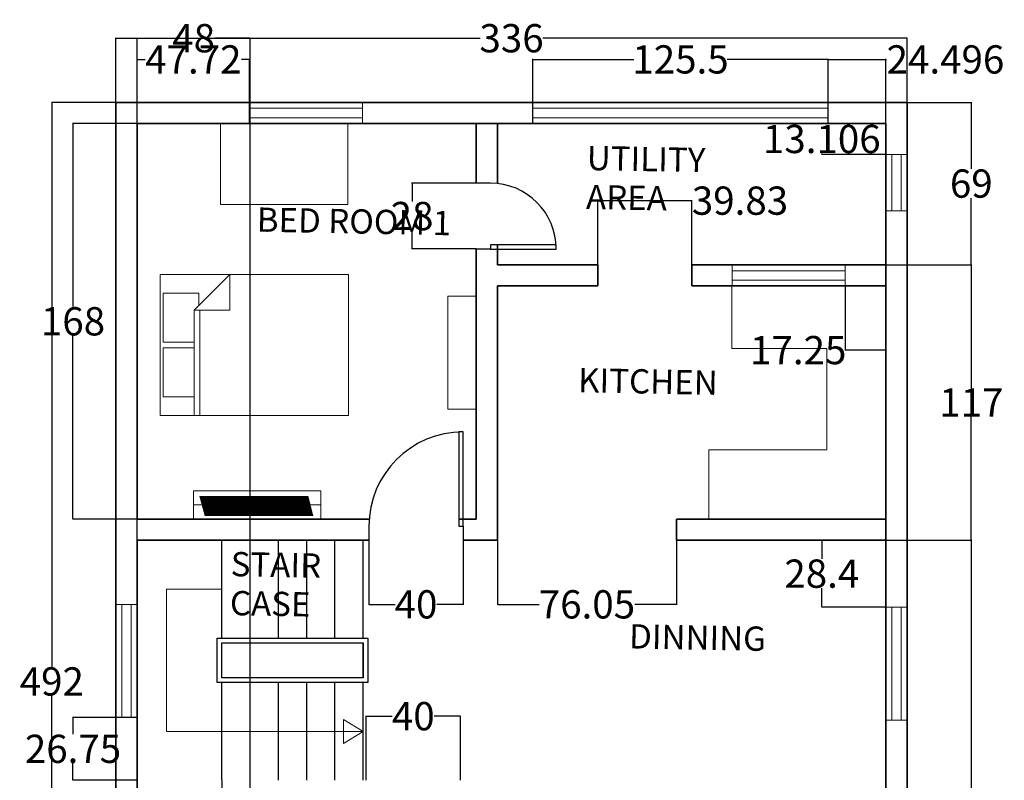
# Model space of a CAD drawing. Units: inches. Extents: x 424 to 1593, y 6 to 578.
# Tile 2 of 4: x 519 to 937, y 255 to 578. Entities that reach past the tile are written whole.
import ezdxf

# ---------------------------------------------------------------- set-up
doc = ezdxf.new("R2010")
doc.units = ezdxf.units.IN
doc.header["$MEASUREMENT"] = 0
for name, color, linetype, lineweight in [('A-ANNO-DIMS', 2, 'Continuous', 18), ('A-ANNO-SYMB', 2, 'Continuous', 18), ('A-AREA-IDEN', 7, 'Continuous', 18), ('A-DOOR', 3, 'Continuous', 25), ('A-FLOR-CASE', 9, 'Continuous', 18), ('A-FLOR-CASE-PATT', 252, 'Continuous', 13), ('A-FLOR-STRS', 7, 'Continuous', 25), ('A-FURN', 8, 'Continuous', 18), ('A-GLAZ', 4, 'Continuous', 18), ('A-WALL', 7, 'Continuous', 35)]:
    doc.layers.add(name, color=color, linetype=linetype, lineweight=lineweight)
doc.styles.get("Standard").update_dxf_attribs({"font": 'arial.ttf'})
doc.dimstyles.get("Standard").update_dxf_attribs({"dimtxt": 12, "dimasz": 0.18, "dimexe": 0.18, "dimexo": 0.0625, "dimgap": 0.09, "dimtad": 0, "dimtih": 1, "dimtoh": 1, "dimdec": 0, "dimzin": 0, "dimdsep": 46, "dimlunit": 3, "dimtxsty": 'Standard', "dimcen": 0.09, "dimadec": 0, "dimazin": 0, "dimtfac": 1, "dimtdec": 0, "dimtofl": 0, "dimtmove": 0, "dimatfit": 3, "dimfxl": 1, "dimtolj": 1, "dimtzin": 0, "dimarcsym": 0})

# ---------------------------------------------------------------- blocks, each defined once
blk = doc.blocks.new('Bed - Queen')
for p, q in [((0, -80.00003), (0, 0)), ((0, 0), (59.99999, 0)), ((59.99999, 0), (59.99999, -80.00003)), ((7.99999, -1.2), (28.79998, -1.2)), ((7.99999, -14.4), (7.99999, -1.2)), ((28.79998, -1.2), (28.79998, -14.4)), ((31.19999, -1.2), (51.99999, -1.2)), ((31.19999, -14.4), (31.19999, -1.2)), ((51.99999, -1.2), (51.99999, -16.4)), ((0, -14.4), (44.8, -14.4)), ((59.99999, -29.6), (44.8, -14.4)), ((44.8, -14.4), (44.8, -29.6)), ((51.99999, -16.4), (46.79936, -16.4)), ((44.8, -16.8), (0, -16.8)), ((44.8, -29.6), (59.99999, -29.6)), ((59.99999, -80.00003), (0, -80.00003))]:
    blk.add_line(p, q)
blk = doc.blocks.new('*U3')
for p, q in [((0, 0), (0, -6)), ((-40, 0), (-40, -6))]:
    blk.add_line(p, q)
blk.add_lwpolyline([(0, 0), (0, 40), (-1.75, 40), (-1.75, 0)], close=True)
blk.add_arc((0, 0), 40, 90, 180)
blk = doc.blocks.new('*U5')
for p, q in [((0, 0), (0, 6)), ((28, 0), (28, 6))]:
    blk.add_line(p, q)
blk.add_lwpolyline([(0, 0), (0, -28), (1.75, -28), (1.75, 0)], close=True)
blk.add_arc((0, 0), 28, 270, 0)
blk = doc.blocks.new('WIN-48IN')
for p, q in [((2.5, 48), (2.5, 0)), ((6.5, 48), (6.5, 0))]:
    blk.add_line(p, q)
blk.add_lwpolyline([(0, 48), (9, 48), (9, 0), (0, 0)], close=True)
blk = doc.blocks.new('WIN-24IN')
for p, q in [((2.5, 0), (2.5, 24)), ((6.5, 0), (6.5, 24))]:
    blk.add_line(p, q)
blk.add_lwpolyline([(9, 0), (0, 0), (0, 24), (9, 24)], close=True)
blk = doc.blocks.new('STAIR-RETURN-102IN')
for p, q in [((2, 60.44), (2, 102)), ((14, 60.44), (14, 102)), ((26, 60.44), (26, 102)), ((38, 60.44), (38, 102)), ((50, 60.44), (50, 102)), ((62, 60.44), (62, 102)), ((2, 43.56), (2, 58.44)), ((62, 43.56), (62, 58.44)), ((2, 0), (2, 41.56)), ((14, 0), (14, 41.56)), ((26, 0), (26, 41.56)), ((38, 0), (38, 41.56)), ((50, 0), (50, 41.56)), ((62, 0), (62, 41.56))]:
    blk.add_line(p, q)
for points in [[(0, 60.44), (64, 60.44), (64, 41.56), (0, 41.56)], [(2, 58.44), (62, 58.44), (62, 43.56), (2, 43.56)]]:
    blk.add_lwpolyline(points, close=True)
blk = doc.blocks.new('CASEWORK-48X12')
blk.add_lwpolyline([(12, 48), (0, 48), (0, 0), (12, 0)], close=True)
blk = doc.blocks.new('*D22')
at = {"layer": 'A-ANNO-DIMS', "color": 0, "lineweight": -2, "transparency": 16777216}
for p, q in [((559.72, 542.59), (559.72, 569.96)), ((559.9, 569.78), (714.38, 569.78)), ((895.54, 569.78), (741.05, 569.78)), ((895.72, 542.59), (895.72, 569.96))]:
    blk.add_line(p, q, dxfattribs=at)
at = {"layer": 'A-ANNO-DIMS', "color": 0, "transparency": 16777216}
for points in [[(559.9, 569.81), (559.9, 569.75), (559.72, 569.78)], [(895.54, 569.81), (895.54, 569.75), (895.72, 569.78)]]:
    blk.add_solid(points, dxfattribs=at)
at = {"layer": 'Defpoints', "color": 0, "transparency": 16777216}
for p in [(895.72, 569.78), (559.72, 542.53), (895.72, 542.53)]:
    blk.add_point(p, dxfattribs=at)
at = {"layer": 'A-ANNO-DIMS', "color": 0, "transparency": 16777216, "insert": (727.72, 569.78), "char_height": 12, "attachment_point": 5}
blk.add_mtext('\\A1;336', dxfattribs=at)
blk = doc.blocks.new('*D23')
at = {"layer": 'A-ANNO-DIMS', "color": 0, "lineweight": -2, "transparency": 16777216}
for p, q in [((559.65, 542.53), (532.29, 542.53)), ((532.47, 542.35), (532.47, 302.75)), ((532.47, 50.71), (532.47, 290.31)), ((559.65, 50.53), (532.29, 50.53))]:
    blk.add_line(p, q, dxfattribs=at)
at = {"layer": 'A-ANNO-DIMS', "color": 0, "transparency": 16777216}
for points in [[(532.44, 542.35), (532.5, 542.35), (532.47, 542.53)], [(532.44, 50.71), (532.5, 50.71), (532.47, 50.53)]]:
    blk.add_solid(points, dxfattribs=at)
at = {"layer": 'Defpoints', "color": 0, "transparency": 16777216}
for p in [(532.47, 542.53), (559.72, 542.53), (559.72, 50.53)]:
    blk.add_point(p, dxfattribs=at)
at = {"layer": 'A-ANNO-DIMS', "color": 0, "transparency": 16777216, "insert": (532.47, 296.53), "char_height": 12, "attachment_point": 5}
blk.add_mtext('\\A1;492', dxfattribs=at)
blk = doc.blocks.new('*D27')
at = {"layer": 'A-ANNO-DIMS', "color": 0, "lineweight": -2, "transparency": 16777216}
for p, q in [((568.65, 533.53), (541.29, 533.53)), ((541.47, 533.35), (541.47, 455.75)), ((541.47, 365.71), (541.47, 443.31)), ((568.65, 365.53), (541.29, 365.53))]:
    blk.add_line(p, q, dxfattribs=at)
at = {"layer": 'A-ANNO-DIMS', "color": 0, "transparency": 16777216}
for points in [[(541.44, 533.35), (541.5, 533.35), (541.47, 533.53)], [(541.44, 365.71), (541.5, 365.71), (541.47, 365.53)]]:
    blk.add_solid(points, dxfattribs=at)
at = {"layer": 'Defpoints', "color": 0, "transparency": 16777216}
for p in [(541.47, 533.53), (568.72, 533.53), (568.72, 365.53)]:
    blk.add_point(p, dxfattribs=at)
at = {"layer": 'A-ANNO-DIMS', "color": 0, "transparency": 16777216, "insert": (541.47, 449.53), "char_height": 12, "attachment_point": 5}
blk.add_mtext('\\A1;168', dxfattribs=at)
blk = doc.blocks.new('*D29')
at = {"layer": 'A-ANNO-DIMS', "color": 0, "lineweight": -2, "transparency": 16777216}
for p, q in [((886.78, 356.53), (923.15, 356.53)), ((922.97, 356.35), (922.97, 239.75)), ((922.97, 110.71), (922.97, 227.31)), ((895.78, 110.53), (923.15, 110.53))]:
    blk.add_line(p, q, dxfattribs=at)
at = {"layer": 'A-ANNO-DIMS', "color": 0, "transparency": 16777216}
for points in [[(922.94, 356.35), (923, 356.35), (922.97, 356.53)], [(922.94, 110.71), (923, 110.71), (922.97, 110.53)]]:
    blk.add_solid(points, dxfattribs=at)
at = {"layer": 'Defpoints', "color": 0, "transparency": 16777216}
for p in [(886.72, 356.53), (922.97, 356.53), (895.72, 110.53)]:
    blk.add_point(p, dxfattribs=at)
at = {"layer": 'A-ANNO-DIMS', "color": 0, "transparency": 16777216, "insert": (922.97, 233.53), "char_height": 12, "attachment_point": 5}
blk.add_mtext('\\A1;246', dxfattribs=at)
blk = doc.blocks.new('*D30')
at = {"layer": 'A-ANNO-DIMS', "color": 0, "lineweight": -2, "transparency": 16777216}
for p, q in [((886.78, 473.53), (923.15, 473.53)), ((922.97, 473.35), (922.97, 421.14)), ((922.97, 356.71), (922.97, 408.92)), ((886.78, 356.53), (923.15, 356.53))]:
    blk.add_line(p, q, dxfattribs=at)
at = {"layer": 'A-ANNO-DIMS', "color": 0, "transparency": 16777216}
for points in [[(922.94, 473.35), (923, 473.35), (922.97, 473.53)], [(922.94, 356.71), (923, 356.71), (922.97, 356.53)]]:
    blk.add_solid(points, dxfattribs=at)
at = {"layer": 'Defpoints', "color": 0, "transparency": 16777216}
for p in [(886.72, 473.53), (922.97, 473.53), (886.72, 356.53)]:
    blk.add_point(p, dxfattribs=at)
at = {"layer": 'A-ANNO-DIMS', "color": 0, "transparency": 16777216, "insert": (922.97, 415.03), "char_height": 12, "attachment_point": 5}
blk.add_mtext('\\A1;117', dxfattribs=at)
blk = doc.blocks.new('*D31')
at = {"layer": 'A-ANNO-DIMS', "color": 0, "lineweight": -2, "transparency": 16777216}
for p, q in [((895.78, 542.53), (923.15, 542.53)), ((922.97, 542.35), (922.97, 514.25)), ((922.97, 473.71), (922.97, 501.81)), ((886.78, 473.53), (923.15, 473.53))]:
    blk.add_line(p, q, dxfattribs=at)
at = {"layer": 'A-ANNO-DIMS', "color": 0, "transparency": 16777216}
for points in [[(922.94, 542.35), (923, 542.35), (922.97, 542.53)], [(922.94, 473.71), (923, 473.71), (922.97, 473.53)]]:
    blk.add_solid(points, dxfattribs=at)
at = {"layer": 'Defpoints', "color": 0, "transparency": 16777216}
for p in [(895.72, 542.53), (922.97, 542.53), (886.72, 473.53)]:
    blk.add_point(p, dxfattribs=at)
at = {"layer": 'A-ANNO-DIMS', "color": 0, "transparency": 16777216, "insert": (922.97, 508.03), "char_height": 12, "attachment_point": 5}
blk.add_mtext('\\A1;69', dxfattribs=at)
blk = doc.blocks.new('*D32')
at = {"layer": 'A-ANNO-DIMS', "color": 0, "lineweight": -2, "transparency": 16777216}
for p, q in [((568.72, 59.59), (568.72, 569.96)), ((568.9, 569.78), (583.78, 569.78)), ((616.54, 569.78), (601.65, 569.78)), ((616.72, 59.59), (616.72, 569.96))]:
    blk.add_line(p, q, dxfattribs=at)
at = {"layer": 'A-ANNO-DIMS', "color": 0, "transparency": 16777216}
for points in [[(568.9, 569.81), (568.9, 569.75), (568.72, 569.78)], [(616.54, 569.81), (616.54, 569.75), (616.72, 569.78)]]:
    blk.add_solid(points, dxfattribs=at)
at = {"layer": 'Defpoints', "color": 0, "transparency": 16777216}
for p in [(616.72, 569.78), (568.72, 59.53), (616.72, 59.53)]:
    blk.add_point(p, dxfattribs=at)
at = {"layer": 'A-ANNO-DIMS', "color": 0, "transparency": 16777216, "insert": (592.72, 569.78), "char_height": 12, "attachment_point": 5}
blk.add_mtext('\\A1;48', dxfattribs=at)
blk = doc.blocks.new('*D34')
at = {"layer": 'A-ANNO-DIMS', "color": 0, "lineweight": -2, "transparency": 16777216}
for p, q in [((568.72, 254.47), (568.72, 23.1)), ((604.72, 254.47), (604.72, 23.1)), ((568.9, 23.28), (578.04, 23.28)), ((604.54, 23.28), (595.39, 23.28))]:
    blk.add_line(p, q, dxfattribs=at)
at = {"layer": 'A-ANNO-DIMS', "color": 0, "transparency": 16777216}
for points in [[(568.9, 23.31), (568.9, 23.25), (568.72, 23.28)], [(604.54, 23.31), (604.54, 23.25), (604.72, 23.28)]]:
    blk.add_solid(points, dxfattribs=at)
at = {"layer": 'Defpoints', "color": 0, "transparency": 16777216}
for p in [(568.72, 254.53), (604.72, 254.53), (604.72, 23.28)]:
    blk.add_point(p, dxfattribs=at)
at = {"layer": 'A-ANNO-DIMS', "color": 0, "transparency": 16777216, "insert": (586.72, 23.28), "char_height": 12, "attachment_point": 5}
blk.add_mtext('\\A1;36', dxfattribs=at)
blk = doc.blocks.new('*D35')
at = {"layer": 'A-ANNO-DIMS', "color": 0, "lineweight": -2, "transparency": 16777216}
for p, q in [((568.65, 281.28), (541.29, 281.28)), ((541.47, 281.1), (541.47, 274.12)), ((541.47, 254.71), (541.47, 261.69)), ((568.65, 254.53), (541.29, 254.53))]:
    blk.add_line(p, q, dxfattribs=at)
at = {"layer": 'A-ANNO-DIMS', "color": 0, "transparency": 16777216}
for points in [[(541.44, 281.1), (541.5, 281.1), (541.47, 281.28)], [(541.44, 254.71), (541.5, 254.71), (541.47, 254.53)]]:
    blk.add_solid(points, dxfattribs=at)
at = {"layer": 'Defpoints', "color": 0, "transparency": 16777216}
for p in [(541.47, 281.28), (568.72, 281.28), (568.72, 254.53)]:
    blk.add_point(p, dxfattribs=at)
at = {"layer": 'A-ANNO-DIMS', "color": 0, "transparency": 16777216, "insert": (541.47, 267.9), "char_height": 12, "attachment_point": 5}
blk.add_mtext('\\A1;26.75', dxfattribs=at)
blk = doc.blocks.new('*D36')
at = {"layer": 'A-ANNO-DIMS', "color": 0, "lineweight": -2, "transparency": 16777216}
for p, q in [((886.65, 356.53), (859.29, 356.53)), ((859.47, 356.35), (859.47, 348.55)), ((859.47, 328.31), (859.47, 336.11)), ((886.65, 328.13), (859.29, 328.13))]:
    blk.add_line(p, q, dxfattribs=at)
at = {"layer": 'A-ANNO-DIMS', "color": 0, "transparency": 16777216}
for points in [[(859.44, 356.35), (859.5, 356.35), (859.47, 356.53)], [(859.44, 328.31), (859.5, 328.31), (859.47, 328.13)]]:
    blk.add_solid(points, dxfattribs=at)
at = {"layer": 'Defpoints', "color": 0, "transparency": 16777216}
for p in [(859.47, 356.53), (886.72, 356.53), (886.72, 328.13)]:
    blk.add_point(p, dxfattribs=at)
at = {"layer": 'A-ANNO-DIMS', "color": 0, "transparency": 16777216, "insert": (859.47, 342.33), "char_height": 12, "attachment_point": 5}
blk.add_mtext('\\A1;28.4', dxfattribs=at)
blk = doc.blocks.new('*D37')
at = {"layer": 'A-ANNO-DIMS', "color": 0, "lineweight": -2, "transparency": 16777216}
for p, q in [((568.72, 533.59), (568.72, 560.96)), ((568.9, 560.78), (572.06, 560.78)), ((616.26, 560.78), (613.09, 560.78)), ((616.44, 533.59), (616.44, 560.96))]:
    blk.add_line(p, q, dxfattribs=at)
at = {"layer": 'A-ANNO-DIMS', "color": 0, "transparency": 16777216}
for points in [[(568.9, 560.81), (568.9, 560.75), (568.72, 560.78)], [(616.26, 560.81), (616.26, 560.75), (616.44, 560.78)]]:
    blk.add_solid(points, dxfattribs=at)
at = {"layer": 'Defpoints', "color": 0, "transparency": 16777216}
for p in [(616.44, 560.78), (568.72, 533.53), (616.44, 533.53)]:
    blk.add_point(p, dxfattribs=at)
at = {"layer": 'A-ANNO-DIMS', "color": 0, "transparency": 16777216, "insert": (592.58, 560.78), "char_height": 12, "attachment_point": 5}
blk.add_mtext('\\A1;47.72', dxfattribs=at)
blk = doc.blocks.new('*D38')
at = {"layer": 'A-ANNO-DIMS', "color": 0, "lineweight": -2, "transparency": 16777216}
for p, q in [((736.73, 533.59), (736.73, 560.96)), ((736.91, 560.78), (779.66, 560.78)), ((862.04, 560.78), (819.29, 560.78)), ((862.22, 533.59), (862.22, 560.96))]:
    blk.add_line(p, q, dxfattribs=at)
at = {"layer": 'A-ANNO-DIMS', "color": 0, "transparency": 16777216}
for points in [[(736.91, 560.81), (736.91, 560.75), (736.73, 560.78)], [(862.04, 560.81), (862.04, 560.75), (862.22, 560.78)]]:
    blk.add_solid(points, dxfattribs=at)
at = {"layer": 'Defpoints', "color": 0, "transparency": 16777216}
for p in [(862.22, 560.78), (736.73, 533.53), (862.22, 533.53)]:
    blk.add_point(p, dxfattribs=at)
at = {"layer": 'A-ANNO-DIMS', "color": 0, "transparency": 16777216, "insert": (799.48, 560.78), "char_height": 12, "attachment_point": 5}
blk.add_mtext('\\A1;125.5', dxfattribs=at)
blk = doc.blocks.new('*D39')
at = {"layer": 'A-ANNO-DIMS', "color": 0, "lineweight": -2, "transparency": 16777216}
for p, q in [((862.22, 533.59), (862.22, 560.96)), ((862.4, 560.78), (886.54, 560.78)), ((886.72, 533.59), (886.72, 560.96)), ((886.72, 560.78), (886.9, 560.78))]:
    blk.add_line(p, q, dxfattribs=at)
at = {"layer": 'A-ANNO-DIMS', "color": 0, "transparency": 16777216}
for points in [[(862.4, 560.81), (862.4, 560.75), (862.22, 560.78)], [(886.54, 560.81), (886.54, 560.75), (886.72, 560.78)]]:
    blk.add_solid(points, dxfattribs=at)
at = {"layer": 'Defpoints', "color": 0, "transparency": 16777216}
for p in [(886.72, 560.78), (862.22, 533.53), (886.72, 533.53)]:
    blk.add_point(p, dxfattribs=at)
at = {"layer": 'A-ANNO-DIMS', "color": 0, "transparency": 16777216, "insert": (911.99, 560.78), "char_height": 12, "attachment_point": 5}
blk.add_mtext('\\A1;24.496', dxfattribs=at)
blk = doc.blocks.new('*D41')
at = {"layer": 'A-ANNO-DIMS', "color": 0, "lineweight": -2, "transparency": 16777216}
for p, q in [((886.65, 533.53), (859.29, 533.53)), ((859.47, 533.35), (859.47, 533.2)), ((886.65, 520.42), (859.29, 520.42)), ((859.47, 520.6), (859.47, 520.76))]:
    blk.add_line(p, q, dxfattribs=at)
at = {"layer": 'A-ANNO-DIMS', "color": 0, "transparency": 16777216}
for points in [[(859.44, 533.35), (859.5, 533.35), (859.47, 533.53)], [(859.44, 520.6), (859.5, 520.6), (859.47, 520.42)]]:
    blk.add_solid(points, dxfattribs=at)
at = {"layer": 'Defpoints', "color": 0, "transparency": 16777216}
for p in [(859.47, 533.53), (886.72, 533.53), (886.72, 520.42)]:
    blk.add_point(p, dxfattribs=at)
at = {"layer": 'A-ANNO-DIMS', "color": 0, "transparency": 16777216, "insert": (859.47, 526.98), "char_height": 12, "attachment_point": 5}
blk.add_mtext('\\A1;13.106', dxfattribs=at)
blk = doc.blocks.new('*D42')
at = {"layer": 'A-ANNO-DIMS', "color": 0, "lineweight": -2, "transparency": 16777216}
for p, q in [((869.47, 464.47), (869.47, 437.1)), ((886.72, 464.47), (886.72, 437.1)), ((869.47, 437.28), (869.29, 437.28)), ((886.54, 437.28), (869.65, 437.28))]:
    blk.add_line(p, q, dxfattribs=at)
at = {"layer": 'A-ANNO-DIMS', "color": 0, "transparency": 16777216}
for points in [[(869.65, 437.31), (869.65, 437.25), (869.47, 437.28)], [(886.54, 437.31), (886.54, 437.25), (886.72, 437.28)]]:
    blk.add_solid(points, dxfattribs=at)
at = {"layer": 'Defpoints', "color": 0, "transparency": 16777216}
for p in [(869.47, 464.53), (886.72, 464.53), (869.47, 437.28)]:
    blk.add_point(p, dxfattribs=at)
at = {"layer": 'A-ANNO-DIMS', "color": 0, "transparency": 16777216, "insert": (849.47, 437.28), "char_height": 12, "attachment_point": 5}
blk.add_mtext('\\A1;17.25', dxfattribs=at)
blk = doc.blocks.new('*D43')
at = {"layer": 'A-ANNO-DIMS', "color": 0, "lineweight": -2, "transparency": 16777216}
for p, q in [((764.39, 473.59), (764.39, 500.96)), ((764.57, 500.78), (804.04, 500.78)), ((804.22, 473.59), (804.22, 500.96)), ((804.22, 500.78), (804.4, 500.78))]:
    blk.add_line(p, q, dxfattribs=at)
at = {"layer": 'A-ANNO-DIMS', "color": 0, "transparency": 16777216}
for points in [[(764.57, 500.81), (764.57, 500.75), (764.39, 500.78)], [(804.04, 500.81), (804.04, 500.75), (804.22, 500.78)]]:
    blk.add_solid(points, dxfattribs=at)
at = {"layer": 'Defpoints', "color": 0, "transparency": 16777216}
for p in [(804.22, 500.78), (764.39, 473.53), (804.22, 473.53)]:
    blk.add_point(p, dxfattribs=at)
at = {"layer": 'A-ANNO-DIMS', "color": 0, "transparency": 16777216, "insert": (824.73, 500.78), "char_height": 12, "attachment_point": 5}
blk.add_mtext('\\A1;39.83', dxfattribs=at)
blk = doc.blocks.new('*D44')
at = {"layer": 'A-ANNO-DIMS', "color": 0, "lineweight": -2, "transparency": 16777216}
for p, q in [((721.72, 356.47), (721.72, 329.1)), ((797.76, 356.47), (797.76, 329.1)), ((721.9, 329.28), (739.41, 329.28)), ((797.58, 329.28), (780.07, 329.28))]:
    blk.add_line(p, q, dxfattribs=at)
at = {"layer": 'A-ANNO-DIMS', "color": 0, "transparency": 16777216}
for points in [[(721.9, 329.31), (721.9, 329.25), (721.72, 329.28)], [(797.58, 329.31), (797.58, 329.25), (797.76, 329.28)]]:
    blk.add_solid(points, dxfattribs=at)
at = {"layer": 'Defpoints', "color": 0, "transparency": 16777216}
for p in [(721.72, 356.53), (797.76, 356.53), (721.72, 329.28)]:
    blk.add_point(p, dxfattribs=at)
at = {"layer": 'A-ANNO-DIMS', "color": 0, "transparency": 16777216, "insert": (759.74, 329.28), "char_height": 12, "attachment_point": 5}
blk.add_mtext('\\A1;76.05', dxfattribs=at)
blk = doc.blocks.new('*D45')
at = {"layer": 'A-ANNO-DIMS', "color": 0, "lineweight": -2, "transparency": 16777216}
for p, q in [((712.65, 508.24), (685.29, 508.24)), ((685.47, 508.06), (685.47, 500.45)), ((685.47, 480.42), (685.47, 488.02)), ((712.65, 480.24), (685.29, 480.24))]:
    blk.add_line(p, q, dxfattribs=at)
at = {"layer": 'A-ANNO-DIMS', "color": 0, "transparency": 16777216}
for points in [[(685.44, 508.06), (685.5, 508.06), (685.47, 508.24)], [(685.44, 480.42), (685.5, 480.42), (685.47, 480.24)]]:
    blk.add_solid(points, dxfattribs=at)
at = {"layer": 'Defpoints', "color": 0, "transparency": 16777216}
for p in [(685.47, 508.24), (712.72, 508.24), (712.72, 480.24)]:
    blk.add_point(p, dxfattribs=at)
at = {"layer": 'A-ANNO-DIMS', "color": 0, "transparency": 16777216, "insert": (685.47, 494.24), "char_height": 12, "attachment_point": 5}
blk.add_mtext('\\A1;28', dxfattribs=at)
blk = doc.blocks.new('*D46')
at = {"layer": 'A-ANNO-DIMS', "color": 0, "lineweight": -2, "transparency": 16777216}
for p, q in [((667.15, 356.47), (667.15, 329.1)), ((707.15, 356.47), (707.15, 329.1)), ((667.33, 329.28), (678.24, 329.28)), ((706.97, 329.28), (696.05, 329.28))]:
    blk.add_line(p, q, dxfattribs=at)
at = {"layer": 'A-ANNO-DIMS', "color": 0, "transparency": 16777216}
for points in [[(667.33, 329.31), (667.33, 329.25), (667.15, 329.28)], [(706.97, 329.31), (706.97, 329.25), (707.15, 329.28)]]:
    blk.add_solid(points, dxfattribs=at)
at = {"layer": 'Defpoints', "color": 0, "transparency": 16777216}
for p in [(667.15, 356.53), (707.15, 356.53), (667.15, 329.28)]:
    blk.add_point(p, dxfattribs=at)
at = {"layer": 'A-ANNO-DIMS', "color": 0, "transparency": 16777216, "insert": (687.15, 329.28), "char_height": 12, "attachment_point": 5}
blk.add_mtext('\\A1;40', dxfattribs=at)
blk = doc.blocks.new('*D47')
at = {"layer": 'A-ANNO-DIMS', "color": 0, "lineweight": -2, "transparency": 16777216}
for p, q in [((666, 254.59), (666, 281.96)), ((666.18, 281.78), (677.09, 281.78)), ((705.82, 281.78), (694.9, 281.78)), ((706, 254.59), (706, 281.96))]:
    blk.add_line(p, q, dxfattribs=at)
at = {"layer": 'A-ANNO-DIMS', "color": 0, "transparency": 16777216}
for points in [[(666.18, 281.81), (666.18, 281.75), (666, 281.78)], [(705.82, 281.81), (705.82, 281.75), (706, 281.78)]]:
    blk.add_solid(points, dxfattribs=at)
at = {"layer": 'Defpoints', "color": 0, "transparency": 16777216}
for p in [(706, 281.78), (666, 254.53), (706, 254.53)]:
    blk.add_point(p, dxfattribs=at)
at = {"layer": 'A-ANNO-DIMS', "color": 0, "transparency": 16777216, "insert": (686, 281.78), "char_height": 12, "attachment_point": 5}
blk.add_mtext('\\A1;40', dxfattribs=at)

msp = doc.modelspace()

# ---------------------------------------------------------------- hatches: boundary and pattern name
at = {"layer": 'A-FLOR-CASE-PATT'}
h = msp.add_hatch(dxfattribs=at)
h.set_pattern_fill('ANSI31', color=256, scale=0.876872, angle=59.407, style=0)
h.paths.add_polyline_path([(595.3414, 375.2477), (597.4788, 366.927), (643.4701, 366.927), (641.3327, 375.2477)])

# ---------------------------------------------------------------- linework, layer by layer
at = {"layer": 'A-ANNO-SYMB'}
for p, q in [((604.7159, 335.7514), (581.2345, 335.7514)), ((581.2345, 335.7514), (581.2345, 275.3079)), ((656.3964, 275.3079), (656.3964, 280.3079)), ((656.3964, 280.3079), (664.7159, 275.3079)), ((581.2345, 275.3079), (656.3421, 275.3079)), ((656.3421, 275.3079), (656.3421, 270.1906)), ((656.3421, 270.1906), (664.7159, 275.3079)), ((664.7159, 275.3079), (656.3964, 275.3079))]:
    msp.add_line(p, q, dxfattribs=at)
at = {"layer": 'A-FLOR-CASE'}
for p, q in [((821.2658, 437.9036), (821.2658, 464.5296)), ((861.6619, 437.9036), (821.2658, 437.9036)), ((861.6619, 394.9418), (861.6619, 437.9036)), ((811.4926, 365.5296), (811.4926, 394.9418)), ((811.4926, 394.9418), (861.6619, 394.9418)), ((592.7159, 371.5296), (646.7159, 371.5296))]:
    msp.add_line(p, q, dxfattribs=at)
for points in [[(604.1046, 533.5296), (658.1746, 533.5296), (658.1746, 499.0792), (604.1046, 499.0792)], [(592.7159, 365.5296), (646.7159, 365.5296), (646.7159, 377.5296), (592.7159, 377.5296)]]:
    msp.add_lwpolyline(points, close=True, dxfattribs=at)
at = {"layer": 'A-GLAZ'}
for p, q in [((736.7307, 540.0296), (862.2197, 540.0296)), ((736.7307, 536.0296), (862.2197, 536.0296))]:
    msp.add_line(p, q, dxfattribs=at)
msp.add_lwpolyline([(736.7307, 533.5296), (736.7307, 542.5296), (862.2197, 542.5296), (862.2197, 533.5296)], close=True, dxfattribs=at)
at = {"layer": 'A-WALL'}
for p, q in [((568.7159, 533.5296), (886.7159, 533.5296)), ((568.7159, 365.5296), (568.7159, 533.5296)), ((712.7159, 508.2372), (712.7159, 533.5296)), ((721.7159, 508.0761), (721.7159, 533.5296)), ((886.7159, 533.5296), (886.7159, 110.5296)), ((721.7159, 473.5296), (721.7159, 481.9872)), ((712.7159, 365.5296), (712.7159, 480.2372)), ((712.7159, 480.2372), (712.7159, 474.2372)), ((721.7159, 473.5296), (764.3852, 473.5296)), ((764.3852, 473.5296), (764.3852, 464.5296)), ((804.2159, 473.5296), (804.2159, 464.5296)), ((804.2159, 473.5296), (886.7159, 473.5296)), ((721.7159, 464.5296), (764.3852, 464.5296)), ((721.7159, 356.5296), (721.7159, 464.5296)), ((804.2159, 464.5296), (886.7159, 464.5296)), ((568.7159, 365.5296), (667.2598, 365.5296)), ((705.3972, 365.5296), (712.7159, 365.5296)), ((797.7624, 365.5296), (886.7159, 365.5296)), ((797.7624, 365.5296), (797.7624, 356.5296)), ((568.7159, 356.5296), (667.1472, 356.5296)), ((568.7159, 254.5296), (568.7159, 356.5296)), ((707.1472, 356.5296), (713.1472, 356.5296)), ((707.1472, 356.5296), (721.7159, 356.5296)), ((797.7624, 356.5296), (886.7159, 356.5296))]:
    msp.add_line(p, q, dxfattribs=at)
msp.add_lwpolyline([(721.7159, 50.5296), (559.7159, 50.5296), (559.7159, 542.5296), (895.7159, 542.5296), (895.7159, 110.5296)], dxfattribs=at)

# ---------------------------------------------------------------- block references
at = {"layer": 'A-DOOR', "rotation": 90}
msp.add_blockref('*U5', (718.7159, 480.2372), dxfattribs=at)
at = {"layer": 'A-DOOR'}
msp.add_blockref('*U3', (707.1472, 362.5296), dxfattribs=at)
at = {"layer": 'A-FLOR-CASE'}
msp.add_blockref('CASEWORK-48X12', (700.716, 412.266), dxfattribs=at)
at = {"layer": 'A-FURN', "rotation": 90}
msp.add_blockref('Bed - Queen', (578.5402, 409.4579), dxfattribs=at)
at = {"layer": 'A-GLAZ'}
for p, rotation in [((664.4386, 533.5297), 90.00000000000024), ((869.466, 464.5297), 89.99999999999991)]:
    msp.add_blockref('WIN-48IN', p, dxfattribs=dict(at, rotation=rotation))
for name, p in [('WIN-24IN', (886.7154, 496.4237)), ('WIN-48IN', (559.716, 281.28)), ('WIN-48IN', (886.716, 280.1297))]:
    msp.add_blockref(name, p, dxfattribs=at)

# ---------------------------------------------------------------- texts
at = {"layer": 'A-AREA-IDEN'}
for s, p in [('UTILITY', (759.6006, 513.7861)), ('AREA', (759.2873, 497.2323)), ('BED ROOM 1', (619.4547, 487.6128)), ('KITCHEN', (755.9049, 419.3717)), ('DINNING', (777.5629, 310.5783))]:
    msp.add_text(s, height=10.30671, rotation=358.915866, dxfattribs=at).set_placement(p)

# ---------------------------------------------------------------- dimensions: what is measured, and where the dimension line sits
at = {"layer": 'A-ANNO-DIMS'}
for base, p1, p2, override, picture, middle in [((895.7159, 569.7796), (559.7159, 542.5296), (895.7159, 542.5296), {"dimdec": 0, "dimlfac": 1, "dimrnd": 0, "dimzin": 0, "dimdsep": 46, "dimlunit": 2}, '*D22', (727.7159, 569.7796)), ((616.4385, 560.7796), (568.7159, 533.5296), (616.4385, 533.5296), {"dimdec": 2, "dimlfac": 1, "dimrnd": 0, "dimzin": 0, "dimdsep": 46, "dimlunit": 2}, '*D37', (592.5772, 560.7796)), ((862.2197, 560.7796), (736.7307, 533.5296), (862.2197, 533.5296), {"dimdec": 1, "dimlfac": 1, "dimrnd": 0, "dimzin": 0, "dimdsep": 46, "dimlunit": 2}, '*D38', (799.4752, 560.7796)), ((886.7159, 560.7796), (862.2197, 533.5296), (886.7159, 533.5296), {"dimdec": 3, "dimlfac": 1, "dimrnd": 0, "dimzin": 0, "dimdsep": 46, "dimlunit": 2}, '*D39', (911.9927, 560.7796)), ((804.2159, 500.7796), (764.3852, 473.5296), (804.2159, 473.5296), {"dimdec": 2, "dimlfac": 1, "dimrnd": 0, "dimzin": 0, "dimdsep": 46, "dimlunit": 2}, '*D43', (824.7288, 500.7796)), ((705.9977, 281.7796), (665.9977, 254.5296), (705.9977, 254.5296), {"dimdec": 0, "dimlfac": 1, "dimrnd": 0, "dimzin": 0, "dimdsep": 46, "dimlunit": 2}, '*D47', (685.9977, 281.7796)), ((604.7159, 23.2796), (568.7159, 254.5296), (604.7159, 254.5296), {"dimdec": 0, "dimlfac": 1, "dimrnd": 0, "dimzin": 0, "dimdsep": 46, "dimlunit": 2}, '*D34', (586.7159, 23.2796))]:
    dim = msp.add_linear_dim(base=base, p1=p1, p2=p2, dimstyle='Standard', override=override, dxfattribs=at)
    dim.commit()
    dim.dimension.update_dxf_attribs({"geometry": picture, "text_midpoint": middle})
for base, p1, p2, angle, override, picture, middle in [((532.4659, 542.5296), (559.7159, 50.5296), (559.7159, 542.5296), 90, {"dimdec": 0, "dimlfac": 1, "dimrnd": 0, "dimzin": 0, "dimdsep": 46, "dimlunit": 2}, '*D23', (532.4659, 296.5296)), ((922.9659, 542.5296), (886.7159, 473.5296), (895.7159, 542.5296), 90, {"dimdec": 0, "dimlfac": 1, "dimrnd": 0, "dimzin": 0, "dimdsep": 46, "dimlunit": 2}, '*D31', (922.9659, 508.0296)), ((541.4659, 533.5296), (568.7159, 365.5296), (568.7159, 533.5296), 90, {"dimdec": 0, "dimlfac": 1, "dimrnd": 0, "dimzin": 0, "dimdsep": 46, "dimlunit": 2}, '*D27', (541.4659, 449.5296)), ((859.4659, 533.5296), (886.7159, 520.4236), (886.7159, 533.5296), 90, {"dimdec": 3, "dimlfac": 1, "dimrnd": 0, "dimzin": 0, "dimdsep": 46, "dimlunit": 2}, '*D41', (859.4659, 526.9766)), ((685.4659, 508.2372), (712.7159, 480.2372), (712.7159, 508.2372), 90, {"dimdec": 0, "dimlfac": 1, "dimrnd": 0, "dimzin": 0, "dimdsep": 46, "dimlunit": 2}, '*D45', (685.4659, 494.2372)), ((922.9659, 473.5296), (886.7159, 356.5296), (886.7159, 473.5296), 90, {"dimdec": 0, "dimlfac": 1, "dimrnd": 0, "dimzin": 0, "dimdsep": 46, "dimlunit": 2}, '*D30', (922.9659, 415.0296)), ((869.4659, 437.2796), (886.7159, 464.5296), (869.4659, 464.5296), 180, {"dimdec": 2, "dimlfac": 1, "dimrnd": 0, "dimzin": 0, "dimdsep": 46, "dimlunit": 2}, '*D42', (849.4688, 437.2796)), ((667.1472, 329.2796), (707.1472, 356.5296), (667.1472, 356.5296), 180, {"dimdec": 0, "dimlfac": 1, "dimrnd": 0, "dimzin": 0, "dimdsep": 46, "dimlunit": 2}, '*D46', (687.1472, 329.2796)), ((721.7159, 329.2796), (797.7624, 356.5296), (721.7159, 356.5296), 180, {"dimdec": 2, "dimlfac": 1, "dimrnd": 0, "dimzin": 0, "dimdsep": 46, "dimlunit": 2}, '*D44', (759.7392, 329.2796)), ((859.4659, 356.5296), (886.7159, 328.1298), (886.7159, 356.5296), 90, {"dimdec": 1, "dimlfac": 1, "dimrnd": 0, "dimzin": 0, "dimdsep": 46, "dimlunit": 2}, '*D36', (859.4659, 342.3297)), ((922.9659, 356.5296), (895.7159, 110.5296), (886.7159, 356.5296), 90, {"dimdec": 0, "dimlfac": 1, "dimrnd": 0, "dimzin": 0, "dimdsep": 46, "dimlunit": 2}, '*D29', (922.9659, 233.5296)), ((541.4659, 281.2801), (568.7159, 254.5296), (568.7159, 281.2801), 90, {"dimdec": 2, "dimlfac": 1, "dimrnd": 0, "dimzin": 0, "dimdsep": 46, "dimlunit": 2}, '*D35', (541.4659, 267.9049))]:
    dim = msp.add_linear_dim(base=base, p1=p1, p2=p2, angle=angle, dimstyle='Standard', override=override, dxfattribs=at)
    dim.commit()
    dim.dimension.update_dxf_attribs({"geometry": picture, "text_midpoint": middle})

# ---------------------------------------------------------------- next in the draw order: wipeouts: each hides what was drawn before it
msp.add_wipeout([(605.3312, 337.5488), (654.1085, 336.6258), (654.4466, 354.4955), (605.6693, 355.4186)]).dxf.layer = 'A-AREA-IDEN'

# ---------------------------------------------------------------- next in the draw order: texts
at = {"layer": 'A-AREA-IDEN'}
msp.add_text('STAIR', height=10.30671, rotation=358.915866, dxfattribs=at).set_placement((608.3627, 341.2753))

# ---------------------------------------------------------------- next in the draw order: wipeouts: each hides what was drawn before it
msp.add_wipeout([(605.0882, 320.9937), (650.0135, 320.1435), (650.3516, 338.0132), (605.4263, 338.8634)]).dxf.layer = 'A-AREA-IDEN'

# ---------------------------------------------------------------- next in the draw order: block references
at = {"layer": 'A-FLOR-STRS'}
msp.add_blockref('STAIR-RETURN-102IN', (602.716, 254.53), dxfattribs=at)

# ---------------------------------------------------------------- next in the draw order: texts
at = {"layer": 'A-AREA-IDEN'}
msp.add_text('CASE', height=10.30671, rotation=358.915866, dxfattribs=at).set_placement((608.0495, 324.7214))

# ---------------------------------------------------------------- next in the draw order: dimensions: what is measured, and where the dimension line sits
at = {"layer": 'A-ANNO-DIMS'}
dim = msp.add_linear_dim(base=(616.7159, 569.7796), p1=(568.7159, 59.5296), p2=(616.7159, 59.5296), dimstyle='Standard', override={"dimdec": 0, "dimlfac": 1, "dimrnd": 0, "dimzin": 0, "dimdsep": 46, "dimlunit": 2}, dxfattribs=at)
dim.commit()
dim.dimension.update_dxf_attribs({"geometry": '*D32', "text_midpoint": (592.7159, 569.7796)})

doc.saveas('drawing.dxf')
